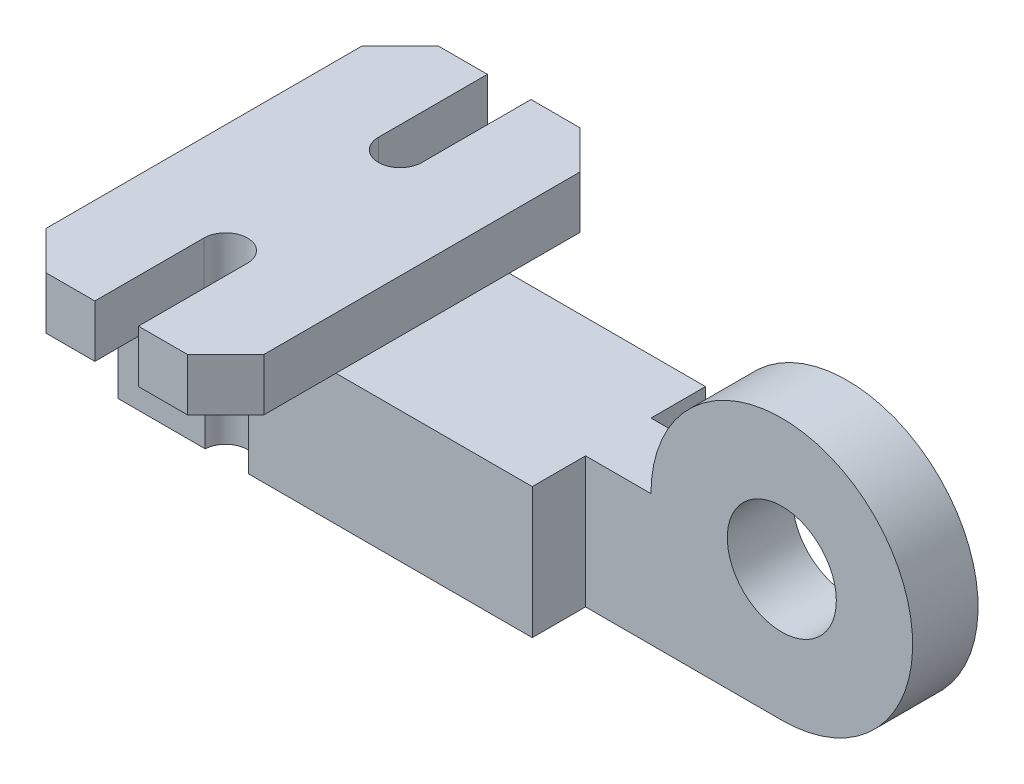
ISO-10303-21;
HEADER;
FILE_DESCRIPTION(('STEP AP214'),'2;1');
FILE_NAME('part.step','',(''),(''),'','','');
FILE_SCHEMA(('AUTOMOTIVE_DESIGN { 1 0 10303 214 1 1 1 1 }'));
ENDSEC;
DATA;
#1=APPLICATION_CONTEXT('core data for automotive mechanical design processes');
#2=APPLICATION_PROTOCOL_DEFINITION('international standard','automotive_design',2000,#1);
#3=PRODUCT_CONTEXT('',#1,'mechanical');
#4=PRODUCT('Part','Part','',(#3));
#5=PRODUCT_RELATED_PRODUCT_CATEGORY('part','',(#4));
#6=PRODUCT_DEFINITION_FORMATION('','',#4);
#7=PRODUCT_DEFINITION_CONTEXT('part definition',#1,'design');
#8=PRODUCT_DEFINITION('design','',#6,#7);
#9=PRODUCT_DEFINITION_SHAPE('','',#8);
#10=(LENGTH_UNIT() NAMED_UNIT(*) SI_UNIT(.MILLI.,.METRE.));
#11=(NAMED_UNIT(*) PLANE_ANGLE_UNIT() SI_UNIT($,.RADIAN.));
#12=(NAMED_UNIT(*) SI_UNIT($,.STERADIAN.) SOLID_ANGLE_UNIT());
#13=UNCERTAINTY_MEASURE_WITH_UNIT(LENGTH_MEASURE(1.E-05),#10,'distance_accuracy_value','');
#14=(GEOMETRIC_REPRESENTATION_CONTEXT(3) GLOBAL_UNCERTAINTY_ASSIGNED_CONTEXT((#13)) GLOBAL_UNIT_ASSIGNED_CONTEXT((#10,
#11,#12)) REPRESENTATION_CONTEXT('',''));
#15=CARTESIAN_POINT('',(0.,0.,0.));
#16=DIRECTION('',(0.,0.,1.));
#17=DIRECTION('',(1.,0.,0.));
#18=AXIS2_PLACEMENT_3D('',#15,#16,#17);
#19=CARTESIAN_POINT('',(0.,30.,7.5));
#20=DIRECTION('',(0.,0.,-1.));
#21=DIRECTION('',(-1.,0.,0.));
#22=AXIS2_PLACEMENT_3D('',#19,#20,#21);
#23=PLANE('',#22);
#24=CARTESIAN_POINT('',(140.,30.,7.5));
#25=DIRECTION('',(0.,0.,1.));
#26=DIRECTION('',(1.,0.,0.));
#27=AXIS2_PLACEMENT_3D('',#24,#25,#26);
#28=CIRCLE('',#27,12.5);
#29=CARTESIAN_POINT('',(152.5,30.,7.5));
#30=VERTEX_POINT('',#29);
#31=EDGE_CURVE('E1012',#30,#30,#28,.T.);
#32=ORIENTED_EDGE('',*,*,#31,.F.);
#33=EDGE_LOOP('',(#32));
#34=FACE_BOUND('',#33,.T.);
#35=DIRECTION('',(1.,0.,0.));
#36=VECTOR('',#35,1.);
#37=CARTESIAN_POINT('',(0.,0.,7.5));
#38=LINE('',#37,#36);
#39=CARTESIAN_POINT('',(95.,0.,7.5));
#40=VERTEX_POINT('',#39);
#41=CARTESIAN_POINT('',(140.,0.,7.5));
#42=VERTEX_POINT('',#41);
#43=EDGE_CURVE('E282',#40,#42,#38,.T.);
#44=ORIENTED_EDGE('',*,*,#43,.T.);
#45=CARTESIAN_POINT('',(140.,30.,7.5));
#46=DIRECTION('',(0.,0.,1.));
#47=DIRECTION('',(1.,0.,0.));
#48=AXIS2_PLACEMENT_3D('',#45,#46,#47);
#49=CIRCLE('',#48,30.);
#50=CARTESIAN_POINT('',(110.,30.,7.5));
#51=VERTEX_POINT('',#50);
#52=EDGE_CURVE('E267',#42,#51,#49,.T.);
#53=ORIENTED_EDGE('',*,*,#52,.T.);
#54=DIRECTION('',(1.,0.,0.));
#55=VECTOR('',#54,1.);
#56=CARTESIAN_POINT('',(0.,30.,7.5));
#57=LINE('',#56,#55);
#58=CARTESIAN_POINT('',(95.,30.,7.5));
#59=VERTEX_POINT('',#58);
#60=EDGE_CURVE('E416',#59,#51,#57,.T.);
#61=ORIENTED_EDGE('',*,*,#60,.F.);
#62=DIRECTION('',(0.,-1.,0.));
#63=VECTOR('',#62,1.);
#64=CARTESIAN_POINT('',(95.,30.,7.5));
#65=LINE('',#64,#63);
#66=EDGE_CURVE('E297',#59,#40,#65,.T.);
#67=ORIENTED_EDGE('',*,*,#66,.T.);
#68=EDGE_LOOP('',(#44,#53,#61,#67));
#69=FACE_BOUND('',#68,.T.);
#70=ADVANCED_FACE('F74',(#34,#69),#23,.F.);
#71=CARTESIAN_POINT('',(0.,30.,-7.5));
#72=DIRECTION('',(0.,0.,-1.));
#73=DIRECTION('',(-1.,0.,0.));
#74=AXIS2_PLACEMENT_3D('',#71,#72,#73);
#75=PLANE('',#74);
#76=CARTESIAN_POINT('',(140.,30.,-7.5));
#77=DIRECTION('',(0.,0.,1.));
#78=DIRECTION('',(1.,0.,0.));
#79=AXIS2_PLACEMENT_3D('',#76,#77,#78);
#80=CIRCLE('',#79,12.5);
#81=CARTESIAN_POINT('',(152.5,30.,-7.5));
#82=VERTEX_POINT('',#81);
#83=EDGE_CURVE('E279',#82,#82,#80,.T.);
#84=ORIENTED_EDGE('',*,*,#83,.T.);
#85=EDGE_LOOP('',(#84));
#86=FACE_BOUND('',#85,.T.);
#87=CARTESIAN_POINT('',(140.,30.,-7.5));
#88=DIRECTION('',(0.,0.,1.));
#89=DIRECTION('',(1.,0.,0.));
#90=AXIS2_PLACEMENT_3D('',#87,#88,#89);
#91=CIRCLE('',#90,30.);
#92=CARTESIAN_POINT('',(140.,0.,-7.5));
#93=VERTEX_POINT('',#92);
#94=CARTESIAN_POINT('',(110.,30.,-7.5));
#95=VERTEX_POINT('',#94);
#96=EDGE_CURVE('E259',#93,#95,#91,.T.);
#97=ORIENTED_EDGE('',*,*,#96,.F.);
#98=DIRECTION('',(1.,0.,0.));
#99=VECTOR('',#98,1.);
#100=CARTESIAN_POINT('',(0.,0.,-7.5));
#101=LINE('',#100,#99);
#102=CARTESIAN_POINT('',(95.,0.,-7.5));
#103=VERTEX_POINT('',#102);
#104=EDGE_CURVE('E263',#103,#93,#101,.T.);
#105=ORIENTED_EDGE('',*,*,#104,.F.);
#106=DIRECTION('',(0.,-1.,0.));
#107=VECTOR('',#106,1.);
#108=CARTESIAN_POINT('',(95.,30.,-7.5));
#109=LINE('',#108,#107);
#110=CARTESIAN_POINT('',(95.,30.,-7.5));
#111=VERTEX_POINT('',#110);
#112=EDGE_CURVE('E298',#111,#103,#109,.T.);
#113=ORIENTED_EDGE('',*,*,#112,.F.);
#114=DIRECTION('',(1.,0.,0.));
#115=VECTOR('',#114,1.);
#116=CARTESIAN_POINT('',(0.,30.,-7.5));
#117=LINE('',#116,#115);
#118=EDGE_CURVE('E264',#111,#95,#117,.T.);
#119=ORIENTED_EDGE('',*,*,#118,.T.);
#120=EDGE_LOOP('',(#97,#105,#113,#119));
#121=FACE_BOUND('',#120,.T.);
#122=ADVANCED_FACE('F261',(#86,#121),#75,.T.);
#123=CARTESIAN_POINT('',(20.,42.,0.));
#124=DIRECTION('',(1.,0.,0.));
#125=DIRECTION('',(0.,0.,-1.));
#126=AXIS2_PLACEMENT_3D('',#123,#124,#125);
#127=PLANE('',#126);
#128=DIRECTION('',(0.,-1.,0.));
#129=VECTOR('',#128,1.);
#130=CARTESIAN_POINT('',(20.,42.,45.));
#131=LINE('',#130,#129);
#132=CARTESIAN_POINT('',(20.,42.,45.));
#133=VERTEX_POINT('',#132);
#134=CARTESIAN_POINT('',(20.,30.,45.));
#135=VERTEX_POINT('',#134);
#136=EDGE_CURVE('E344',#133,#135,#131,.T.);
#137=ORIENTED_EDGE('',*,*,#136,.T.);
#138=DIRECTION('',(0.,0.,-1.));
#139=VECTOR('',#138,1.);
#140=CARTESIAN_POINT('',(20.,30.,0.));
#141=LINE('',#140,#139);
#142=CARTESIAN_POINT('',(20.,30.,20.));
#143=VERTEX_POINT('',#142);
#144=EDGE_CURVE('E406',#135,#143,#141,.T.);
#145=ORIENTED_EDGE('',*,*,#144,.T.);
#146=DIRECTION('',(0.,-1.,0.));
#147=VECTOR('',#146,1.);
#148=CARTESIAN_POINT('',(20.,42.,20.));
#149=LINE('',#148,#147);
#150=CARTESIAN_POINT('',(20.,42.,20.));
#151=VERTEX_POINT('',#150);
#152=EDGE_CURVE('E85',#151,#143,#149,.T.);
#153=ORIENTED_EDGE('',*,*,#152,.F.);
#154=DIRECTION('',(0.,0.,1.));
#155=VECTOR('',#154,1.);
#156=CARTESIAN_POINT('',(20.,42.,0.));
#157=LINE('',#156,#155);
#158=EDGE_CURVE('E301',#151,#133,#157,.T.);
#159=ORIENTED_EDGE('',*,*,#158,.T.);
#160=EDGE_LOOP('',(#137,#145,#153,#159));
#161=FACE_BOUND('',#160,.T.);
#162=ADVANCED_FACE('F78',(#161),#127,.T.);
#163=CARTESIAN_POINT('',(25.,42.,20.));
#164=DIRECTION('',(0.,-1.,0.));
#165=DIRECTION('',(0.,0.,-1.));
#166=AXIS2_PLACEMENT_3D('',#163,#164,#165);
#167=CYLINDRICAL_SURFACE('',#166,5.);
#168=CARTESIAN_POINT('',(25.,30.,20.));
#169=DIRECTION('',(0.,-1.,0.));
#170=DIRECTION('',(0.,0.,-1.));
#171=AXIS2_PLACEMENT_3D('',#168,#169,#170);
#172=CIRCLE('',#171,5.);
#173=CARTESIAN_POINT('',(30.,30.,20.));
#174=VERTEX_POINT('',#173);
#175=CARTESIAN_POINT('',(29.9917789461064,30.,19.7133940802973));
#176=VERTEX_POINT('',#175);
#177=EDGE_CURVE('E411',#174,#176,#172,.F.);
#178=ORIENTED_EDGE('',*,*,#177,.F.);
#179=DIRECTION('',(0.,-1.,0.));
#180=VECTOR('',#179,1.);
#181=CARTESIAN_POINT('',(30.,42.,20.));
#182=LINE('',#181,#180);
#183=CARTESIAN_POINT('',(30.,42.,20.));
#184=VERTEX_POINT('',#183);
#185=EDGE_CURVE('E392',#184,#174,#182,.T.);
#186=ORIENTED_EDGE('',*,*,#185,.F.);
#187=CARTESIAN_POINT('',(25.,42.,20.));
#188=DIRECTION('',(0.,1.,0.));
#189=DIRECTION('',(0.,0.,1.));
#190=AXIS2_PLACEMENT_3D('',#187,#188,#189);
#191=CIRCLE('',#190,5.);
#192=EDGE_CURVE('E308',#151,#184,#191,.F.);
#193=ORIENTED_EDGE('',*,*,#192,.F.);
#194=ORIENTED_EDGE('',*,*,#152,.T.);
#195=CARTESIAN_POINT('',(20.0082210538936,30.,19.7133940802973));
#196=VERTEX_POINT('',#195);
#197=EDGE_CURVE('E401',#196,#143,#172,.F.);
#198=ORIENTED_EDGE('',*,*,#197,.F.);
#199=DIRECTION('',(0.,-1.,0.));
#200=VECTOR('',#199,1.);
#201=CARTESIAN_POINT('',(20.0082210538936,42.,19.7133940802973));
#202=LINE('',#201,#200);
#203=CARTESIAN_POINT('',(20.0082210538936,0.,19.7133940802973));
#204=VERTEX_POINT('',#203);
#205=EDGE_CURVE('E492',#196,#204,#202,.T.);
#206=ORIENTED_EDGE('',*,*,#205,.T.);
#207=CARTESIAN_POINT('',(25.,0.,20.));
#208=DIRECTION('',(0.,1.,0.));
#209=DIRECTION('',(0.,0.,1.));
#210=AXIS2_PLACEMENT_3D('',#207,#208,#209);
#211=CIRCLE('',#210,5.);
#212=CARTESIAN_POINT('',(29.9917789461064,0.,19.7133940802973));
#213=VERTEX_POINT('',#212);
#214=EDGE_CURVE('E305',#204,#213,#211,.F.);
#215=ORIENTED_EDGE('',*,*,#214,.T.);
#216=DIRECTION('',(0.,-1.,0.));
#217=VECTOR('',#216,1.);
#218=CARTESIAN_POINT('',(29.9917789461064,42.,19.7133940802973));
#219=LINE('',#218,#217);
#220=EDGE_CURVE('E494',#213,#176,#219,.F.);
#221=ORIENTED_EDGE('',*,*,#220,.T.);
#222=EDGE_LOOP('',(#178,#186,#193,#194,#198,#206,#215,#221));
#223=FACE_BOUND('',#222,.T.);
#224=ADVANCED_FACE('F402',(#223),#167,.F.);
#225=CARTESIAN_POINT('',(30.,42.,0.));
#226=DIRECTION('',(1.,0.,0.));
#227=DIRECTION('',(0.,0.,-1.));
#228=AXIS2_PLACEMENT_3D('',#225,#226,#227);
#229=PLANE('',#228);
#230=DIRECTION('',(0.,0.,-1.));
#231=VECTOR('',#230,1.);
#232=CARTESIAN_POINT('',(30.,30.,0.));
#233=LINE('',#232,#231);
#234=CARTESIAN_POINT('',(30.,30.,45.));
#235=VERTEX_POINT('',#234);
#236=EDGE_CURVE('E443',#235,#174,#233,.T.);
#237=ORIENTED_EDGE('',*,*,#236,.F.);
#238=DIRECTION('',(0.,-1.,0.));
#239=VECTOR('',#238,1.);
#240=CARTESIAN_POINT('',(30.,42.,45.));
#241=LINE('',#240,#239);
#242=CARTESIAN_POINT('',(30.,42.,45.));
#243=VERTEX_POINT('',#242);
#244=EDGE_CURVE('E393',#243,#235,#241,.T.);
#245=ORIENTED_EDGE('',*,*,#244,.F.);
#246=DIRECTION('',(0.,0.,1.));
#247=VECTOR('',#246,1.);
#248=CARTESIAN_POINT('',(30.,42.,0.));
#249=LINE('',#248,#247);
#250=EDGE_CURVE('E310',#184,#243,#249,.T.);
#251=ORIENTED_EDGE('',*,*,#250,.F.);
#252=ORIENTED_EDGE('',*,*,#185,.T.);
#253=EDGE_LOOP('',(#237,#245,#251,#252));
#254=FACE_BOUND('',#253,.T.);
#255=ADVANCED_FACE('F633',(#254),#229,.F.);
#256=CARTESIAN_POINT('',(0.,42.,45.));
#257=DIRECTION('',(0.,0.,-1.));
#258=DIRECTION('',(-1.,0.,0.));
#259=AXIS2_PLACEMENT_3D('',#256,#257,#258);
#260=PLANE('',#259);
#261=DIRECTION('',(-1.,0.,0.));
#262=VECTOR('',#261,1.);
#263=CARTESIAN_POINT('',(123.,30.,45.));
#264=LINE('',#263,#262);
#265=CARTESIAN_POINT('',(41.197317330942,30.,45.));
#266=VERTEX_POINT('',#265);
#267=EDGE_CURVE('E463',#266,#235,#264,.T.);
#268=ORIENTED_EDGE('',*,*,#267,.F.);
#269=DIRECTION('',(0.,-1.,0.));
#270=VECTOR('',#269,1.);
#271=CARTESIAN_POINT('',(41.197317330942,42.,45.));
#272=LINE('',#271,#270);
#273=CARTESIAN_POINT('',(41.197317330942,42.,45.));
#274=VERTEX_POINT('',#273);
#275=EDGE_CURVE('E389',#274,#266,#272,.T.);
#276=ORIENTED_EDGE('',*,*,#275,.F.);
#277=DIRECTION('',(1.,0.,0.));
#278=VECTOR('',#277,1.);
#279=CARTESIAN_POINT('',(0.,42.,45.));
#280=LINE('',#279,#278);
#281=EDGE_CURVE('E313',#243,#274,#280,.T.);
#282=ORIENTED_EDGE('',*,*,#281,.F.);
#283=ORIENTED_EDGE('',*,*,#244,.T.);
#284=EDGE_LOOP('',(#268,#276,#282,#283));
#285=FACE_BOUND('',#284,.T.);
#286=ADVANCED_FACE('F458',(#285),#260,.F.);
#287=CARTESIAN_POINT('',(43.0986586654707,42.,43.0986586654713));
#288=DIRECTION('',(0.707106781186543,0.,0.707106781186552));
#289=DIRECTION('',(0.707106781186552,0.,-0.707106781186543));
#290=AXIS2_PLACEMENT_3D('',#287,#288,#289);
#291=PLANE('',#290);
#292=ORIENTED_EDGE('',*,*,#275,.T.);
#293=DIRECTION('',(0.707106781186552,0.,-0.707106781186543));
#294=VECTOR('',#293,1.);
#295=CARTESIAN_POINT('',(43.0986586654707,30.,43.0986586654713));
#296=LINE('',#295,#294);
#297=CARTESIAN_POINT('',(50.,30.,36.1973173309421));
#298=VERTEX_POINT('',#297);
#299=EDGE_CURVE('E436',#266,#298,#296,.T.);
#300=ORIENTED_EDGE('',*,*,#299,.T.);
#301=DIRECTION('',(0.,-1.,0.));
#302=VECTOR('',#301,1.);
#303=CARTESIAN_POINT('',(50.,42.,36.1973173309421));
#304=LINE('',#303,#302);
#305=CARTESIAN_POINT('',(50.,42.,36.1973173309421));
#306=VERTEX_POINT('',#305);
#307=EDGE_CURVE('E384',#306,#298,#304,.T.);
#308=ORIENTED_EDGE('',*,*,#307,.F.);
#309=DIRECTION('',(-0.707106781186552,0.,0.707106781186543));
#310=VECTOR('',#309,1.);
#311=CARTESIAN_POINT('',(43.0986586654707,42.,43.0986586654713));
#312=LINE('',#311,#310);
#313=EDGE_CURVE('E311',#306,#274,#312,.T.);
#314=ORIENTED_EDGE('',*,*,#313,.T.);
#315=EDGE_LOOP('',(#292,#300,#308,#314));
#316=FACE_BOUND('',#315,.T.);
#317=ADVANCED_FACE('F445',(#316),#291,.T.);
#318=CARTESIAN_POINT('',(50.,42.,0.));
#319=DIRECTION('',(1.,0.,0.));
#320=DIRECTION('',(0.,0.,-1.));
#321=AXIS2_PLACEMENT_3D('',#318,#319,#320);
#322=PLANE('',#321);
#323=ORIENTED_EDGE('',*,*,#307,.T.);
#324=DIRECTION('',(0.,0.,1.));
#325=VECTOR('',#324,1.);
#326=CARTESIAN_POINT('',(50.,30.,0.));
#327=LINE('',#326,#325);
#328=CARTESIAN_POINT('',(50.,30.,19.7133940802973));
#329=VERTEX_POINT('',#328);
#330=EDGE_CURVE('E428',#329,#298,#327,.T.);
#331=ORIENTED_EDGE('',*,*,#330,.F.);
#332=CARTESIAN_POINT('',(50.,30.,-20.));
#333=VERTEX_POINT('',#332);
#334=EDGE_CURVE('E300',#333,#329,#327,.T.);
#335=ORIENTED_EDGE('',*,*,#334,.F.);
#336=DIRECTION('',(0.,0.,1.));
#337=VECTOR('',#336,1.);
#338=CARTESIAN_POINT('',(50.,30.,0.));
#339=LINE('',#338,#337);
#340=CARTESIAN_POINT('',(50.,30.,-36.1973173309421));
#341=VERTEX_POINT('',#340);
#342=EDGE_CURVE('E506',#341,#333,#339,.T.);
#343=ORIENTED_EDGE('',*,*,#342,.F.);
#344=DIRECTION('',(0.,-1.,0.));
#345=VECTOR('',#344,1.);
#346=CARTESIAN_POINT('',(50.,42.,-36.1973173309421));
#347=LINE('',#346,#345);
#348=CARTESIAN_POINT('',(50.,42.,-36.1973173309421));
#349=VERTEX_POINT('',#348);
#350=EDGE_CURVE('E385',#349,#341,#347,.T.);
#351=ORIENTED_EDGE('',*,*,#350,.F.);
#352=DIRECTION('',(0.,0.,1.));
#353=VECTOR('',#352,1.);
#354=CARTESIAN_POINT('',(50.,42.,0.));
#355=LINE('',#354,#353);
#356=EDGE_CURVE('E316',#349,#306,#355,.T.);
#357=ORIENTED_EDGE('',*,*,#356,.T.);
#358=EDGE_LOOP('',(#323,#331,#335,#343,#351,#357));
#359=FACE_BOUND('',#358,.T.);
#360=ADVANCED_FACE('F446',(#359),#322,.T.);
#361=CARTESIAN_POINT('',(0.,42.,0.));
#362=DIRECTION('',(-1.,0.,0.));
#363=DIRECTION('',(0.,0.,1.));
#364=AXIS2_PLACEMENT_3D('',#361,#362,#363);
#365=PLANE('',#364);
#366=DIRECTION('',(0.,-1.,0.));
#367=VECTOR('',#366,1.);
#368=CARTESIAN_POINT('',(0.,0.,19.7133940802973));
#369=LINE('',#368,#367);
#370=CARTESIAN_POINT('',(0.,30.,19.7133940802973));
#371=VERTEX_POINT('',#370);
#372=CARTESIAN_POINT('',(0.,0.,19.7133940802973));
#373=VERTEX_POINT('',#372);
#374=EDGE_CURVE('E90',#371,#373,#369,.T.);
#375=ORIENTED_EDGE('',*,*,#374,.F.);
#376=DIRECTION('',(0.,0.,1.));
#377=VECTOR('',#376,1.);
#378=CARTESIAN_POINT('',(0.,30.,0.));
#379=LINE('',#378,#377);
#380=CARTESIAN_POINT('',(0.,30.,36.197317330942));
#381=VERTEX_POINT('',#380);
#382=EDGE_CURVE('E482',#371,#381,#379,.T.);
#383=ORIENTED_EDGE('',*,*,#382,.T.);
#384=DIRECTION('',(0.,-1.,0.));
#385=VECTOR('',#384,1.);
#386=CARTESIAN_POINT('',(0.,42.,36.197317330942));
#387=LINE('',#386,#385);
#388=CARTESIAN_POINT('',(0.,42.,36.197317330942));
#389=VERTEX_POINT('',#388);
#390=EDGE_CURVE('E356',#389,#381,#387,.T.);
#391=ORIENTED_EDGE('',*,*,#390,.F.);
#392=DIRECTION('',(0.,0.,-1.));
#393=VECTOR('',#392,1.);
#394=CARTESIAN_POINT('',(0.,42.,0.));
#395=LINE('',#394,#393);
#396=CARTESIAN_POINT('',(0.,42.,-36.197317330942));
#397=VERTEX_POINT('',#396);
#398=EDGE_CURVE('E336',#389,#397,#395,.T.);
#399=ORIENTED_EDGE('',*,*,#398,.T.);
#400=DIRECTION('',(0.,-1.,0.));
#401=VECTOR('',#400,1.);
#402=CARTESIAN_POINT('',(0.,42.,-36.197317330942));
#403=LINE('',#402,#401);
#404=CARTESIAN_POINT('',(0.,30.,-36.197317330942));
#405=VERTEX_POINT('',#404);
#406=EDGE_CURVE('E363',#397,#405,#403,.T.);
#407=ORIENTED_EDGE('',*,*,#406,.T.);
#408=DIRECTION('',(0.,0.,-1.));
#409=VECTOR('',#408,1.);
#410=CARTESIAN_POINT('',(0.,30.,0.));
#411=LINE('',#410,#409);
#412=CARTESIAN_POINT('',(0.,30.,-20.));
#413=VERTEX_POINT('',#412);
#414=EDGE_CURVE('E479',#413,#405,#411,.T.);
#415=ORIENTED_EDGE('',*,*,#414,.F.);
#416=DIRECTION('',(0.,1.,0.));
#417=VECTOR('',#416,1.);
#418=CARTESIAN_POINT('',(0.,0.,-20.));
#419=LINE('',#418,#417);
#420=CARTESIAN_POINT('',(0.,0.,-20.));
#421=VERTEX_POINT('',#420);
#422=EDGE_CURVE('E268',#421,#413,#419,.T.);
#423=ORIENTED_EDGE('',*,*,#422,.F.);
#424=DIRECTION('',(0.,0.,-1.));
#425=VECTOR('',#424,1.);
#426=CARTESIAN_POINT('',(0.,0.,0.));
#427=LINE('',#426,#425);
#428=EDGE_CURVE('E307',#373,#421,#427,.T.);
#429=ORIENTED_EDGE('',*,*,#428,.F.);
#430=EDGE_LOOP('',(#375,#383,#391,#399,#407,#415,#423,#429));
#431=FACE_BOUND('',#430,.T.);
#432=ADVANCED_FACE('F528',(#431),#365,.T.);
#433=CARTESIAN_POINT('',(-18.098658665471,42.,18.098658665471));
#434=DIRECTION('',(0.707106781186549,0.,-0.707106781186546));
#435=DIRECTION('',(-0.707106781186546,0.,-0.707106781186549));
#436=AXIS2_PLACEMENT_3D('',#433,#434,#435);
#437=PLANE('',#436);
#438=DIRECTION('',(-0.707106781186546,0.,-0.707106781186549));
#439=VECTOR('',#438,1.);
#440=CARTESIAN_POINT('',(-18.098658665471,30.,18.098658665471));
#441=LINE('',#440,#439);
#442=CARTESIAN_POINT('',(8.80268266905791,30.,45.));
#443=VERTEX_POINT('',#442);
#444=EDGE_CURVE('E448',#443,#381,#441,.T.);
#445=ORIENTED_EDGE('',*,*,#444,.F.);
#446=DIRECTION('',(0.,-1.,0.));
#447=VECTOR('',#446,1.);
#448=CARTESIAN_POINT('',(8.80268266905791,42.,45.));
#449=LINE('',#448,#447);
#450=CARTESIAN_POINT('',(8.80268266905791,42.,45.));
#451=VERTEX_POINT('',#450);
#452=EDGE_CURVE('E354',#451,#443,#449,.T.);
#453=ORIENTED_EDGE('',*,*,#452,.F.);
#454=DIRECTION('',(0.707106781186546,0.,0.707106781186549));
#455=VECTOR('',#454,1.);
#456=CARTESIAN_POINT('',(-18.098658665471,42.,18.098658665471));
#457=LINE('',#456,#455);
#458=EDGE_CURVE('E343',#389,#451,#457,.T.);
#459=ORIENTED_EDGE('',*,*,#458,.F.);
#460=ORIENTED_EDGE('',*,*,#390,.T.);
#461=EDGE_LOOP('',(#445,#453,#459,#460));
#462=FACE_BOUND('',#461,.T.);
#463=ADVANCED_FACE('F533',(#462),#437,.F.);
#464=CARTESIAN_POINT('',(0.,42.,45.));
#465=DIRECTION('',(0.,0.,-1.));
#466=DIRECTION('',(-1.,0.,0.));
#467=AXIS2_PLACEMENT_3D('',#464,#465,#466);
#468=PLANE('',#467);
#469=EDGE_CURVE('E462',#135,#443,#264,.T.);
#470=ORIENTED_EDGE('',*,*,#469,.F.);
#471=ORIENTED_EDGE('',*,*,#136,.F.);
#472=DIRECTION('',(1.,0.,0.));
#473=VECTOR('',#472,1.);
#474=CARTESIAN_POINT('',(0.,42.,45.));
#475=LINE('',#474,#473);
#476=EDGE_CURVE('E341',#451,#133,#475,.T.);
#477=ORIENTED_EDGE('',*,*,#476,.F.);
#478=ORIENTED_EDGE('',*,*,#452,.T.);
#479=EDGE_LOOP('',(#470,#471,#477,#478));
#480=FACE_BOUND('',#479,.T.);
#481=ADVANCED_FACE('F602',(#480),#468,.F.);
#482=CARTESIAN_POINT('',(43.0986586654707,42.,-43.0986586654713));
#483=DIRECTION('',(-0.707106781186543,0.,0.707106781186552));
#484=DIRECTION('',(0.707106781186552,0.,0.707106781186543));
#485=AXIS2_PLACEMENT_3D('',#482,#483,#484);
#486=PLANE('',#485);
#487=ORIENTED_EDGE('',*,*,#350,.T.);
#488=DIRECTION('',(-0.707106781186552,0.,-0.707106781186543));
#489=VECTOR('',#488,1.);
#490=CARTESIAN_POINT('',(43.0986586654707,30.,-43.0986586654713));
#491=LINE('',#490,#489);
#492=CARTESIAN_POINT('',(41.197317330942,30.,-45.));
#493=VERTEX_POINT('',#492);
#494=EDGE_CURVE('E504',#341,#493,#491,.T.);
#495=ORIENTED_EDGE('',*,*,#494,.T.);
#496=DIRECTION('',(0.,-1.,0.));
#497=VECTOR('',#496,1.);
#498=CARTESIAN_POINT('',(41.197317330942,42.,-45.));
#499=LINE('',#498,#497);
#500=CARTESIAN_POINT('',(41.197317330942,42.,-45.));
#501=VERTEX_POINT('',#500);
#502=EDGE_CURVE('E377',#501,#493,#499,.T.);
#503=ORIENTED_EDGE('',*,*,#502,.F.);
#504=DIRECTION('',(-0.707106781186552,0.,-0.707106781186543));
#505=VECTOR('',#504,1.);
#506=CARTESIAN_POINT('',(43.0986586654707,42.,-43.0986586654713));
#507=LINE('',#506,#505);
#508=EDGE_CURVE('E317',#349,#501,#507,.T.);
#509=ORIENTED_EDGE('',*,*,#508,.F.);
#510=EDGE_LOOP('',(#487,#495,#503,#509));
#511=FACE_BOUND('',#510,.T.);
#512=ADVANCED_FACE('F568',(#511),#486,.F.);
#513=CARTESIAN_POINT('',(0.,42.,-45.));
#514=DIRECTION('',(0.,0.,-1.));
#515=DIRECTION('',(-1.,0.,0.));
#516=AXIS2_PLACEMENT_3D('',#513,#514,#515);
#517=PLANE('',#516);
#518=DIRECTION('',(-1.,0.,0.));
#519=VECTOR('',#518,1.);
#520=CARTESIAN_POINT('',(123.,30.,-45.));
#521=LINE('',#520,#519);
#522=CARTESIAN_POINT('',(30.,30.,-45.));
#523=VERTEX_POINT('',#522);
#524=EDGE_CURVE('E484',#493,#523,#521,.T.);
#525=ORIENTED_EDGE('',*,*,#524,.T.);
#526=DIRECTION('',(0.,-1.,0.));
#527=VECTOR('',#526,1.);
#528=CARTESIAN_POINT('',(30.,42.,-45.));
#529=LINE('',#528,#527);
#530=CARTESIAN_POINT('',(30.,42.,-45.));
#531=VERTEX_POINT('',#530);
#532=EDGE_CURVE('E376',#531,#523,#529,.T.);
#533=ORIENTED_EDGE('',*,*,#532,.F.);
#534=DIRECTION('',(1.,0.,0.));
#535=VECTOR('',#534,1.);
#536=CARTESIAN_POINT('',(0.,42.,-45.));
#537=LINE('',#536,#535);
#538=EDGE_CURVE('E321',#531,#501,#537,.T.);
#539=ORIENTED_EDGE('',*,*,#538,.T.);
#540=ORIENTED_EDGE('',*,*,#502,.T.);
#541=EDGE_LOOP('',(#525,#533,#539,#540));
#542=FACE_BOUND('',#541,.T.);
#543=ADVANCED_FACE('F571',(#542),#517,.T.);
#544=CARTESIAN_POINT('',(30.,42.,0.));
#545=DIRECTION('',(-1.,0.,0.));
#546=DIRECTION('',(0.,0.,1.));
#547=AXIS2_PLACEMENT_3D('',#544,#545,#546);
#548=PLANE('',#547);
#549=DIRECTION('',(0.,0.,-1.));
#550=VECTOR('',#549,1.);
#551=CARTESIAN_POINT('',(30.,30.,0.));
#552=LINE('',#551,#550);
#553=CARTESIAN_POINT('',(30.,30.,-20.));
#554=VERTEX_POINT('',#553);
#555=EDGE_CURVE('E501',#554,#523,#552,.T.);
#556=ORIENTED_EDGE('',*,*,#555,.F.);
#557=DIRECTION('',(0.,-1.,0.));
#558=VECTOR('',#557,1.);
#559=CARTESIAN_POINT('',(30.,42.,-20.));
#560=LINE('',#559,#558);
#561=CARTESIAN_POINT('',(30.,42.,-20.));
#562=VERTEX_POINT('',#561);
#563=EDGE_CURVE('E373',#562,#554,#560,.T.);
#564=ORIENTED_EDGE('',*,*,#563,.F.);
#565=DIRECTION('',(0.,0.,-1.));
#566=VECTOR('',#565,1.);
#567=CARTESIAN_POINT('',(30.,42.,0.));
#568=LINE('',#567,#566);
#569=EDGE_CURVE('E322',#562,#531,#568,.T.);
#570=ORIENTED_EDGE('',*,*,#569,.T.);
#571=ORIENTED_EDGE('',*,*,#532,.T.);
#572=EDGE_LOOP('',(#556,#564,#570,#571));
#573=FACE_BOUND('',#572,.T.);
#574=ADVANCED_FACE('F580',(#573),#548,.T.);
#575=CARTESIAN_POINT('',(25.,42.,-20.));
#576=DIRECTION('',(0.,-1.,0.));
#577=DIRECTION('',(0.,0.,-1.));
#578=AXIS2_PLACEMENT_3D('',#575,#576,#577);
#579=CYLINDRICAL_SURFACE('',#578,5.);
#580=CARTESIAN_POINT('',(25.,0.,-20.));
#581=DIRECTION('',(0.,1.,0.));
#582=DIRECTION('',(0.,0.,1.));
#583=AXIS2_PLACEMENT_3D('',#580,#581,#582);
#584=CIRCLE('',#583,5.);
#585=CARTESIAN_POINT('',(20.,0.,-20.));
#586=VERTEX_POINT('',#585);
#587=CARTESIAN_POINT('',(30.,0.,-20.));
#588=VERTEX_POINT('',#587);
#589=EDGE_CURVE('E346',#586,#588,#584,.T.);
#590=ORIENTED_EDGE('',*,*,#589,.F.);
#591=DIRECTION('',(0.,1.,0.));
#592=VECTOR('',#591,1.);
#593=CARTESIAN_POINT('',(20.,42.,-20.));
#594=LINE('',#593,#592);
#595=CARTESIAN_POINT('',(20.,30.,-20.));
#596=VERTEX_POINT('',#595);
#597=EDGE_CURVE('E461',#586,#596,#594,.T.);
#598=ORIENTED_EDGE('',*,*,#597,.T.);
#599=DIRECTION('',(0.,-1.,0.));
#600=VECTOR('',#599,1.);
#601=CARTESIAN_POINT('',(20.,42.,-20.));
#602=LINE('',#601,#600);
#603=CARTESIAN_POINT('',(20.,42.,-20.));
#604=VERTEX_POINT('',#603);
#605=EDGE_CURVE('E367',#604,#596,#602,.T.);
#606=ORIENTED_EDGE('',*,*,#605,.F.);
#607=CARTESIAN_POINT('',(25.,42.,-20.));
#608=DIRECTION('',(0.,1.,0.));
#609=DIRECTION('',(0.,0.,1.));
#610=AXIS2_PLACEMENT_3D('',#607,#608,#609);
#611=CIRCLE('',#610,5.);
#612=EDGE_CURVE('E330',#604,#562,#611,.T.);
#613=ORIENTED_EDGE('',*,*,#612,.T.);
#614=ORIENTED_EDGE('',*,*,#563,.T.);
#615=DIRECTION('',(0.,-1.,0.));
#616=VECTOR('',#615,1.);
#617=CARTESIAN_POINT('',(30.,42.,-20.));
#618=LINE('',#617,#616);
#619=EDGE_CURVE('E470',#588,#554,#618,.F.);
#620=ORIENTED_EDGE('',*,*,#619,.F.);
#621=EDGE_LOOP('',(#590,#598,#606,#613,#614,#620));
#622=FACE_BOUND('',#621,.T.);
#623=ADVANCED_FACE('F560',(#622),#579,.F.);
#624=CARTESIAN_POINT('',(20.,42.,0.));
#625=DIRECTION('',(-1.,0.,0.));
#626=DIRECTION('',(0.,0.,1.));
#627=AXIS2_PLACEMENT_3D('',#624,#625,#626);
#628=PLANE('',#627);
#629=ORIENTED_EDGE('',*,*,#605,.T.);
#630=DIRECTION('',(0.,0.,-1.));
#631=VECTOR('',#630,1.);
#632=CARTESIAN_POINT('',(20.,30.,0.));
#633=LINE('',#632,#631);
#634=CARTESIAN_POINT('',(20.,30.,-45.));
#635=VERTEX_POINT('',#634);
#636=EDGE_CURVE('E498',#596,#635,#633,.T.);
#637=ORIENTED_EDGE('',*,*,#636,.T.);
#638=DIRECTION('',(0.,-1.,0.));
#639=VECTOR('',#638,1.);
#640=CARTESIAN_POINT('',(20.,42.,-45.));
#641=LINE('',#640,#639);
#642=CARTESIAN_POINT('',(20.,42.,-45.));
#643=VERTEX_POINT('',#642);
#644=EDGE_CURVE('E370',#643,#635,#641,.T.);
#645=ORIENTED_EDGE('',*,*,#644,.F.);
#646=DIRECTION('',(0.,0.,-1.));
#647=VECTOR('',#646,1.);
#648=CARTESIAN_POINT('',(20.,42.,0.));
#649=LINE('',#648,#647);
#650=EDGE_CURVE('E329',#604,#643,#649,.T.);
#651=ORIENTED_EDGE('',*,*,#650,.F.);
#652=EDGE_LOOP('',(#629,#637,#645,#651));
#653=FACE_BOUND('',#652,.T.);
#654=ADVANCED_FACE('F548',(#653),#628,.F.);
#655=CARTESIAN_POINT('',(0.,42.,-45.));
#656=DIRECTION('',(0.,0.,-1.));
#657=DIRECTION('',(-1.,0.,0.));
#658=AXIS2_PLACEMENT_3D('',#655,#656,#657);
#659=PLANE('',#658);
#660=CARTESIAN_POINT('',(8.80268266905791,30.,-45.));
#661=VERTEX_POINT('',#660);
#662=EDGE_CURVE('E486',#635,#661,#521,.T.);
#663=ORIENTED_EDGE('',*,*,#662,.T.);
#664=DIRECTION('',(0.,-1.,0.));
#665=VECTOR('',#664,1.);
#666=CARTESIAN_POINT('',(8.80268266905791,42.,-45.));
#667=LINE('',#666,#665);
#668=CARTESIAN_POINT('',(8.80268266905791,42.,-45.));
#669=VERTEX_POINT('',#668);
#670=EDGE_CURVE('E365',#669,#661,#667,.T.);
#671=ORIENTED_EDGE('',*,*,#670,.F.);
#672=DIRECTION('',(1.,0.,0.));
#673=VECTOR('',#672,1.);
#674=CARTESIAN_POINT('',(0.,42.,-45.));
#675=LINE('',#674,#673);
#676=EDGE_CURVE('E335',#669,#643,#675,.T.);
#677=ORIENTED_EDGE('',*,*,#676,.T.);
#678=ORIENTED_EDGE('',*,*,#644,.T.);
#679=EDGE_LOOP('',(#663,#671,#677,#678));
#680=FACE_BOUND('',#679,.T.);
#681=ADVANCED_FACE('F544',(#680),#659,.T.);
#682=CARTESIAN_POINT('',(-18.098658665471,42.,-18.098658665471));
#683=DIRECTION('',(-0.707106781186549,0.,-0.707106781186546));
#684=DIRECTION('',(-0.707106781186546,0.,0.707106781186549));
#685=AXIS2_PLACEMENT_3D('',#682,#683,#684);
#686=PLANE('',#685);
#687=DIRECTION('',(0.707106781186546,0.,-0.707106781186549));
#688=VECTOR('',#687,1.);
#689=CARTESIAN_POINT('',(-18.098658665471,30.,-18.098658665471));
#690=LINE('',#689,#688);
#691=EDGE_CURVE('E499',#405,#661,#690,.T.);
#692=ORIENTED_EDGE('',*,*,#691,.F.);
#693=ORIENTED_EDGE('',*,*,#406,.F.);
#694=DIRECTION('',(0.707106781186546,0.,-0.707106781186549));
#695=VECTOR('',#694,1.);
#696=CARTESIAN_POINT('',(-18.098658665471,42.,-18.098658665471));
#697=LINE('',#696,#695);
#698=EDGE_CURVE('E333',#397,#669,#697,.T.);
#699=ORIENTED_EDGE('',*,*,#698,.T.);
#700=ORIENTED_EDGE('',*,*,#670,.T.);
#701=EDGE_LOOP('',(#692,#693,#699,#700));
#702=FACE_BOUND('',#701,.T.);
#703=ADVANCED_FACE('F541',(#702),#686,.T.);
#704=CARTESIAN_POINT('',(0.,42.,0.));
#705=DIRECTION('',(0.,1.,0.));
#706=DIRECTION('',(0.,0.,1.));
#707=AXIS2_PLACEMENT_3D('',#704,#705,#706);
#708=PLANE('',#707);
#709=ORIENTED_EDGE('',*,*,#158,.F.);
#710=ORIENTED_EDGE('',*,*,#192,.T.);
#711=ORIENTED_EDGE('',*,*,#250,.T.);
#712=ORIENTED_EDGE('',*,*,#281,.T.);
#713=ORIENTED_EDGE('',*,*,#313,.F.);
#714=ORIENTED_EDGE('',*,*,#356,.F.);
#715=ORIENTED_EDGE('',*,*,#508,.T.);
#716=ORIENTED_EDGE('',*,*,#538,.F.);
#717=ORIENTED_EDGE('',*,*,#569,.F.);
#718=ORIENTED_EDGE('',*,*,#612,.F.);
#719=ORIENTED_EDGE('',*,*,#650,.T.);
#720=ORIENTED_EDGE('',*,*,#676,.F.);
#721=ORIENTED_EDGE('',*,*,#698,.F.);
#722=ORIENTED_EDGE('',*,*,#398,.F.);
#723=ORIENTED_EDGE('',*,*,#458,.T.);
#724=ORIENTED_EDGE('',*,*,#476,.T.);
#725=EDGE_LOOP('',(#709,#710,#711,#712,#713,#714,#715,#716,#717,#718,#719,#720,#721,#722,#723,#724));
#726=FACE_BOUND('',#725,.T.);
#727=ADVANCED_FACE('F451',(#726),#708,.T.);
#728=CARTESIAN_POINT('',(0.,0.,0.));
#729=DIRECTION('',(0.,1.,0.));
#730=DIRECTION('',(0.,0.,1.));
#731=AXIS2_PLACEMENT_3D('',#728,#729,#730);
#732=PLANE('',#731);
#733=ORIENTED_EDGE('',*,*,#104,.T.);
#734=DIRECTION('',(0.,0.,1.));
#735=VECTOR('',#734,1.);
#736=CARTESIAN_POINT('',(140.,0.,-7.5));
#737=LINE('',#736,#735);
#738=EDGE_CURVE('E275',#93,#42,#737,.T.);
#739=ORIENTED_EDGE('',*,*,#738,.T.);
#740=ORIENTED_EDGE('',*,*,#43,.F.);
#741=DIRECTION('',(0.,0.,-1.));
#742=VECTOR('',#741,1.);
#743=CARTESIAN_POINT('',(95.,0.,0.));
#744=LINE('',#743,#742);
#745=CARTESIAN_POINT('',(95.,0.,19.7133940802973));
#746=VERTEX_POINT('',#745);
#747=EDGE_CURVE('E286',#746,#40,#744,.T.);
#748=ORIENTED_EDGE('',*,*,#747,.F.);
#749=DIRECTION('',(-1.,0.,0.));
#750=VECTOR('',#749,1.);
#751=CARTESIAN_POINT('',(123.,0.,19.7133940802973));
#752=LINE('',#751,#750);
#753=EDGE_CURVE('E467',#746,#213,#752,.T.);
#754=ORIENTED_EDGE('',*,*,#753,.T.);
#755=ORIENTED_EDGE('',*,*,#214,.F.);
#756=EDGE_CURVE('E471',#204,#373,#752,.T.);
#757=ORIENTED_EDGE('',*,*,#756,.T.);
#758=ORIENTED_EDGE('',*,*,#428,.T.);
#759=DIRECTION('',(-1.,0.,0.));
#760=VECTOR('',#759,1.);
#761=CARTESIAN_POINT('',(123.,0.,-20.));
#762=LINE('',#761,#760);
#763=EDGE_CURVE('E485',#586,#421,#762,.T.);
#764=ORIENTED_EDGE('',*,*,#763,.F.);
#765=ORIENTED_EDGE('',*,*,#589,.T.);
#766=DIRECTION('',(-1.,0.,0.));
#767=VECTOR('',#766,1.);
#768=CARTESIAN_POINT('',(0.,0.,-20.));
#769=LINE('',#768,#767);
#770=CARTESIAN_POINT('',(95.,0.,-20.));
#771=VERTEX_POINT('',#770);
#772=EDGE_CURVE('E288',#771,#588,#769,.T.);
#773=ORIENTED_EDGE('',*,*,#772,.F.);
#774=EDGE_CURVE('E281',#103,#771,#744,.T.);
#775=ORIENTED_EDGE('',*,*,#774,.F.);
#776=EDGE_LOOP('',(#733,#739,#740,#748,#754,#755,#757,#758,#764,#765,#773,#775));
#777=FACE_BOUND('',#776,.T.);
#778=ADVANCED_FACE('F283',(#777),#732,.F.);
#779=CARTESIAN_POINT('',(95.,30.,0.));
#780=DIRECTION('',(-1.,0.,0.));
#781=DIRECTION('',(0.,0.,1.));
#782=AXIS2_PLACEMENT_3D('',#779,#780,#781);
#783=PLANE('',#782);
#784=DIRECTION('',(0.,0.,-1.));
#785=VECTOR('',#784,1.);
#786=CARTESIAN_POINT('',(95.,30.,0.));
#787=LINE('',#786,#785);
#788=CARTESIAN_POINT('',(95.,30.,19.7133940802973));
#789=VERTEX_POINT('',#788);
#790=EDGE_CURVE('E295',#789,#59,#787,.T.);
#791=ORIENTED_EDGE('',*,*,#790,.F.);
#792=DIRECTION('',(0.,-1.,0.));
#793=VECTOR('',#792,1.);
#794=CARTESIAN_POINT('',(95.,30.,19.7133940802973));
#795=LINE('',#794,#793);
#796=EDGE_CURVE('E96',#789,#746,#795,.T.);
#797=ORIENTED_EDGE('',*,*,#796,.T.);
#798=ORIENTED_EDGE('',*,*,#747,.T.);
#799=ORIENTED_EDGE('',*,*,#66,.F.);
#800=EDGE_LOOP('',(#791,#797,#798,#799));
#801=FACE_BOUND('',#800,.T.);
#802=ADVANCED_FACE('F520',(#801),#783,.F.);
#803=ORIENTED_EDGE('',*,*,#774,.T.);
#804=DIRECTION('',(0.,-1.,0.));
#805=VECTOR('',#804,1.);
#806=CARTESIAN_POINT('',(95.,30.,-20.));
#807=LINE('',#806,#805);
#808=CARTESIAN_POINT('',(95.,30.,-20.));
#809=VERTEX_POINT('',#808);
#810=EDGE_CURVE('E291',#809,#771,#807,.T.);
#811=ORIENTED_EDGE('',*,*,#810,.F.);
#812=EDGE_CURVE('E420',#111,#809,#787,.T.);
#813=ORIENTED_EDGE('',*,*,#812,.F.);
#814=ORIENTED_EDGE('',*,*,#112,.T.);
#815=EDGE_LOOP('',(#803,#811,#813,#814));
#816=FACE_BOUND('',#815,.T.);
#817=ADVANCED_FACE('F570',(#816),#783,.F.);
#818=CARTESIAN_POINT('',(0.,30.,-20.));
#819=DIRECTION('',(0.,0.,1.));
#820=DIRECTION('',(1.,0.,0.));
#821=AXIS2_PLACEMENT_3D('',#818,#819,#820);
#822=PLANE('',#821);
#823=ORIENTED_EDGE('',*,*,#772,.T.);
#824=ORIENTED_EDGE('',*,*,#619,.T.);
#825=DIRECTION('',(-1.,0.,0.));
#826=VECTOR('',#825,1.);
#827=CARTESIAN_POINT('',(123.,30.,-20.));
#828=LINE('',#827,#826);
#829=EDGE_CURVE('E487',#333,#554,#828,.T.);
#830=ORIENTED_EDGE('',*,*,#829,.F.);
#831=DIRECTION('',(-1.,0.,0.));
#832=VECTOR('',#831,1.);
#833=CARTESIAN_POINT('',(0.,30.,-20.));
#834=LINE('',#833,#832);
#835=EDGE_CURVE('E422',#809,#333,#834,.T.);
#836=ORIENTED_EDGE('',*,*,#835,.F.);
#837=ORIENTED_EDGE('',*,*,#810,.T.);
#838=EDGE_LOOP('',(#823,#824,#830,#836,#837));
#839=FACE_BOUND('',#838,.T.);
#840=ADVANCED_FACE('F559',(#839),#822,.F.);
#841=CARTESIAN_POINT('',(0.,30.,0.));
#842=DIRECTION('',(0.,1.,0.));
#843=DIRECTION('',(0.,0.,1.));
#844=AXIS2_PLACEMENT_3D('',#841,#842,#843);
#845=PLANE('',#844);
#846=DIRECTION('',(-1.,0.,0.));
#847=VECTOR('',#846,1.);
#848=CARTESIAN_POINT('',(0.,30.,19.7133940802973));
#849=LINE('',#848,#847);
#850=EDGE_CURVE('E12',#789,#329,#849,.T.);
#851=ORIENTED_EDGE('',*,*,#850,.F.);
#852=ORIENTED_EDGE('',*,*,#790,.T.);
#853=ORIENTED_EDGE('',*,*,#60,.T.);
#854=DIRECTION('',(0.,0.,1.));
#855=VECTOR('',#854,1.);
#856=CARTESIAN_POINT('',(110.,30.,0.));
#857=LINE('',#856,#855);
#858=EDGE_CURVE('E425',#95,#51,#857,.T.);
#859=ORIENTED_EDGE('',*,*,#858,.F.);
#860=ORIENTED_EDGE('',*,*,#118,.F.);
#861=ORIENTED_EDGE('',*,*,#812,.T.);
#862=ORIENTED_EDGE('',*,*,#835,.T.);
#863=ORIENTED_EDGE('',*,*,#334,.T.);
#864=EDGE_LOOP('',(#851,#852,#853,#859,#860,#861,#862,#863));
#865=FACE_BOUND('',#864,.T.);
#866=ADVANCED_FACE('F519',(#865),#845,.T.);
#867=CARTESIAN_POINT('',(123.,0.,19.7133940802973));
#868=DIRECTION('',(0.,0.,-1.));
#869=DIRECTION('',(0.,1.,0.));
#870=AXIS2_PLACEMENT_3D('',#867,#868,#869);
#871=PLANE('',#870);
#872=ORIENTED_EDGE('',*,*,#753,.F.);
#873=ORIENTED_EDGE('',*,*,#796,.F.);
#874=ORIENTED_EDGE('',*,*,#850,.T.);
#875=DIRECTION('',(-1.,0.,0.));
#876=VECTOR('',#875,1.);
#877=CARTESIAN_POINT('',(123.,30.,19.7133940802973));
#878=LINE('',#877,#876);
#879=EDGE_CURVE('E438',#329,#176,#878,.T.);
#880=ORIENTED_EDGE('',*,*,#879,.T.);
#881=ORIENTED_EDGE('',*,*,#220,.F.);
#882=EDGE_LOOP('',(#872,#873,#874,#880,#881));
#883=FACE_BOUND('',#882,.T.);
#884=ADVANCED_FACE('F509',(#883),#871,.F.);
#885=CARTESIAN_POINT('',(123.,30.,0.));
#886=DIRECTION('',(0.,-1.,0.));
#887=DIRECTION('',(0.,0.,-1.));
#888=AXIS2_PLACEMENT_3D('',#885,#886,#887);
#889=PLANE('',#888);
#890=ORIENTED_EDGE('',*,*,#177,.T.);
#891=ORIENTED_EDGE('',*,*,#879,.F.);
#892=ORIENTED_EDGE('',*,*,#330,.T.);
#893=ORIENTED_EDGE('',*,*,#299,.F.);
#894=ORIENTED_EDGE('',*,*,#267,.T.);
#895=ORIENTED_EDGE('',*,*,#236,.T.);
#896=EDGE_LOOP('',(#890,#891,#892,#893,#894,#895));
#897=FACE_BOUND('',#896,.T.);
#898=ADVANCED_FACE('F434',(#897),#889,.T.);
#899=CARTESIAN_POINT('',(123.,30.,0.));
#900=DIRECTION('',(0.,1.,0.));
#901=DIRECTION('',(0.,0.,1.));
#902=AXIS2_PLACEMENT_3D('',#899,#900,#901);
#903=PLANE('',#902);
#904=ORIENTED_EDGE('',*,*,#342,.T.);
#905=ORIENTED_EDGE('',*,*,#829,.T.);
#906=ORIENTED_EDGE('',*,*,#555,.T.);
#907=ORIENTED_EDGE('',*,*,#524,.F.);
#908=ORIENTED_EDGE('',*,*,#494,.F.);
#909=EDGE_LOOP('',(#904,#905,#906,#907,#908));
#910=FACE_BOUND('',#909,.T.);
#911=ADVANCED_FACE('F576',(#910),#903,.F.);
#912=EDGE_CURVE('E481',#596,#413,#828,.T.);
#913=ORIENTED_EDGE('',*,*,#912,.T.);
#914=ORIENTED_EDGE('',*,*,#414,.T.);
#915=ORIENTED_EDGE('',*,*,#691,.T.);
#916=ORIENTED_EDGE('',*,*,#662,.F.);
#917=ORIENTED_EDGE('',*,*,#636,.F.);
#918=EDGE_LOOP('',(#913,#914,#915,#916,#917));
#919=FACE_BOUND('',#918,.T.);
#920=ADVANCED_FACE('F543',(#919),#903,.F.);
#921=CARTESIAN_POINT('',(123.,0.,-20.));
#922=DIRECTION('',(0.,0.,1.));
#923=DIRECTION('',(1.,0.,0.));
#924=AXIS2_PLACEMENT_3D('',#921,#922,#923);
#925=PLANE('',#924);
#926=ORIENTED_EDGE('',*,*,#763,.T.);
#927=ORIENTED_EDGE('',*,*,#422,.T.);
#928=ORIENTED_EDGE('',*,*,#912,.F.);
#929=ORIENTED_EDGE('',*,*,#597,.F.);
#930=EDGE_LOOP('',(#926,#927,#928,#929));
#931=FACE_BOUND('',#930,.T.);
#932=ADVANCED_FACE('F554',(#931),#925,.F.);
#933=ORIENTED_EDGE('',*,*,#469,.T.);
#934=ORIENTED_EDGE('',*,*,#444,.T.);
#935=ORIENTED_EDGE('',*,*,#382,.F.);
#936=EDGE_CURVE('E474',#196,#371,#878,.T.);
#937=ORIENTED_EDGE('',*,*,#936,.F.);
#938=ORIENTED_EDGE('',*,*,#197,.T.);
#939=ORIENTED_EDGE('',*,*,#144,.F.);
#940=EDGE_LOOP('',(#933,#934,#935,#937,#938,#939));
#941=FACE_BOUND('',#940,.T.);
#942=ADVANCED_FACE('F588',(#941),#889,.T.);
#943=ORIENTED_EDGE('',*,*,#936,.T.);
#944=ORIENTED_EDGE('',*,*,#374,.T.);
#945=ORIENTED_EDGE('',*,*,#756,.F.);
#946=ORIENTED_EDGE('',*,*,#205,.F.);
#947=EDGE_LOOP('',(#943,#944,#945,#946));
#948=FACE_BOUND('',#947,.T.);
#949=ADVANCED_FACE('F657',(#948),#871,.F.);
#950=CARTESIAN_POINT('',(140.,30.,-7.5));
#951=DIRECTION('',(0.,0.,1.));
#952=DIRECTION('',(1.,0.,0.));
#953=AXIS2_PLACEMENT_3D('',#950,#951,#952);
#954=CYLINDRICAL_SURFACE('',#953,30.);
#955=ORIENTED_EDGE('',*,*,#52,.F.);
#956=ORIENTED_EDGE('',*,*,#738,.F.);
#957=ORIENTED_EDGE('',*,*,#96,.T.);
#958=ORIENTED_EDGE('',*,*,#858,.T.);
#959=EDGE_LOOP('',(#955,#956,#957,#958));
#960=FACE_BOUND('',#959,.T.);
#961=ADVANCED_FACE('F272',(#960),#954,.T.);
#962=CARTESIAN_POINT('',(140.,30.,-7.5));
#963=DIRECTION('',(0.,0.,1.));
#964=DIRECTION('',(1.,0.,0.));
#965=AXIS2_PLACEMENT_3D('',#962,#963,#964);
#966=CYLINDRICAL_SURFACE('',#965,12.5);
#967=ORIENTED_EDGE('',*,*,#83,.F.);
#968=EDGE_LOOP('',(#967));
#969=FACE_BOUND('',#968,.T.);
#970=ORIENTED_EDGE('',*,*,#31,.T.);
#971=EDGE_LOOP('',(#970));
#972=FACE_BOUND('',#971,.T.);
#973=ADVANCED_FACE('F907',(#969,#972),#966,.F.);
#974=CLOSED_SHELL('',(#70,#122,#162,#224,#255,#286,#317,#360,#432,#463,#481,#512,#543,#574,#623,
#654,#681,#703,#727,#778,#802,#817,#840,#866,#884,#898,#911,#920,#932,#942,#949,#961,#973));
#975=MANIFOLD_SOLID_BREP('B2',#974);
#976=ADVANCED_BREP_SHAPE_REPRESENTATION('',(#18,#975),#14);
#977=SHAPE_DEFINITION_REPRESENTATION(#9,#976);
ENDSEC;
END-ISO-10303-21;
